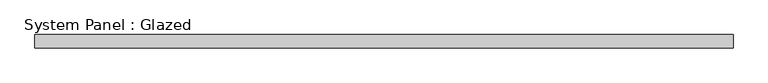
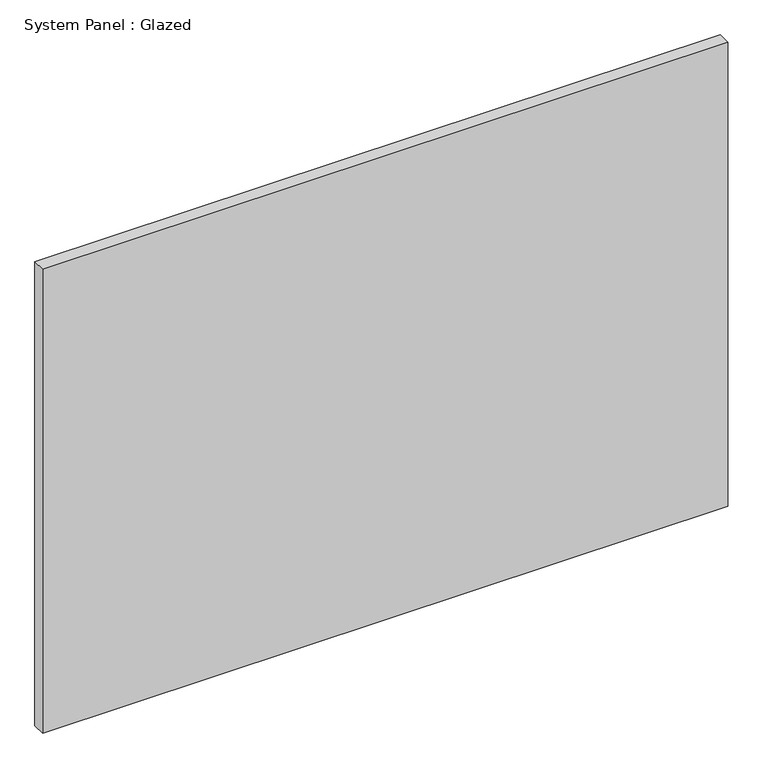
"""IFC4 building model written with IfcOpenShell, lengths in millimetres: plate geometry, System Panel : Glazed."""

from ifc_helpers import new_model, si_unit, origin, origin_with_axes, place, context, project, spatial, polyline, outline, extrude, source, transform, mapped, element, save


def system_panel_glazed_0f6e2381(model_context):
    return source(origin(), model_context, "Body", "SweptSolid", [
        extrude(outline(polyline([(648.3, 24.5), (-648.3, 24.5), (-648.3, 49.5), (648.3, 49.5), (648.3, 24.5)])), origin_with_axes(), (0.0, 0.0, 1.0), 927.5595785),
    ])


if __name__ == "__main__":
    model = new_model("IFC4")
    model_context = context("Model", 3, world=origin())
    ifc_project = project(units=[si_unit("LENGTHUNIT", "METRE", prefix="MILLI")], contexts=[model_context])
    site = spatial("IfcSite", under=ifc_project)
    building = spatial("IfcBuilding", under=site)
    placement = place(None, origin())
    system_panel_glazed_shape = system_panel_glazed_0f6e2381(model_context)
    element("IfcPlate", 1, ObjectType="System Panel : Glazed", at=placement, inside=building, context=model_context, shape_type="MappedRepresentation", body=[
        mapped(system_panel_glazed_shape, transform((0.0, 0.0, 0.0), x_axis=(1.0, 0.0, 0.0), y_axis=(0.0, 1.0, 0.0), z_axis=(0.0, 0.0, 1.0))),
    ])
    save(model, "model.ifc")

# Revit data of these elements
# Type "System Panel : Glazed"
#   Construction Type Id = "GSP4R"
#   Analytic Construction = "1/8 in Pilkington single glazing"
#   Visual Light Transmittance = 0.9
#   Solar Heat Gain Coefficient = 0.86
#   Heat Transfer Coefficient (U) = 6.7069 W/(m²·K)
# Element 1 (IfcPlate, "System Panel : Glazed")
#   Materials on its faces: "Glass"
# Materials
#   "Glass": class "Glass", colour RGB 0 128 192, transparency 0.9, Description = "Soda Lime Glass", Cost = 0
